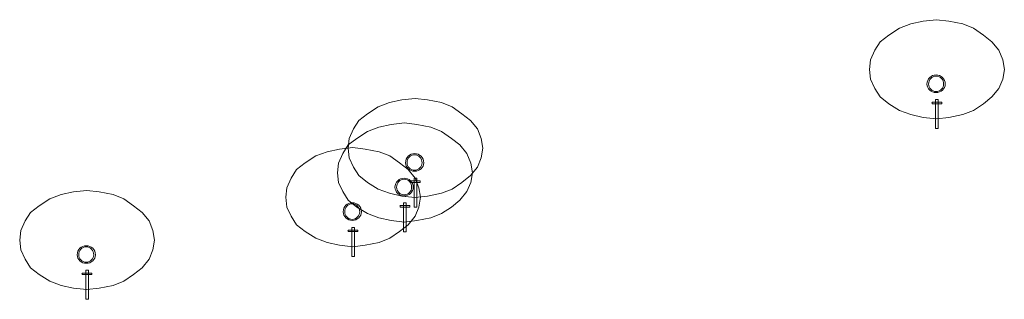
# Model space of a CAD drawing. Units: inches. Extents: x 22042254 to 25404563, y 17568978 to 17626777.
# Tile 45 of 45: x 25402992 to 25404563, y 17598821 to 17599268. Entities that reach past the tile are written whole.
import ezdxf

# ---------------------------------------------------------------- set-up
doc = ezdxf.new("R2010")
doc.units = ezdxf.units.IN
doc.header["$MEASUREMENT"] = 0
doc.layers.add('PLUMBING FIXTURES', color=9, linetype='Continuous', lineweight=18)

# ---------------------------------------------------------------- blocks, each defined once
blk = doc.blocks.new('WASH')
for p, q in [((268674.25, -2306.86), (268674.25, -2306.65)), ((268674.71, -2306.29), (268675.07, -2306.29)), ((268675.53, -2306.86), (268675.53, -2306.65)), ((268674.71, -2310.15), (268675.07, -2310.15))]:
    blk.add_line(p, q)
for points in [[(268665.93, -2302.29), (268666.07, -2301.01), (268666.64, -2299.72), (268667.36, -2298.58), (268668.5, -2297.72), (268669.93, -2296.79), (268671.43, -2296.22), (268673.07, -2295.86), (268674.86, -2295.65), (268676.5, -2295.86), (268678.36, -2296.22), (268679.78, -2296.79), (268681.07, -2297.72), (268682.21, -2298.58), (268683.14, -2299.72), (268683.64, -2301.01), (268683.86, -2302.29), (268683.64, -2303.58), (268683.14, -2304.79), (268682.21, -2305.94), (268681.07, -2306.86), (268679.78, -2307.72), (268678.36, -2308.29), (268676.5, -2308.65), (268674.86, -2308.86), (268673.07, -2308.65), (268671.43, -2308.29), (268669.93, -2307.72), (268668.5, -2306.86), (268667.36, -2305.94), (268666.64, -2304.79), (268666.07, -2303.58)], [(268674.14, -2306.65), (268674.14, -2306.65)], [(268674.86, -2306.29), (268674.86, -2306.29)], [(268675.43, -2306.65), (268675.43, -2306.65)]]:
    blk.add_lwpolyline(points, close=True)
for points in [[(268674.25, -2306.65), (268675.53, -2306.65), (268675.53, -2306.65)], [(268674.25, -2306.86), (268675.53, -2306.86), (268675.53, -2306.86)], [(268674.71, -2310.15), (268674.71, -2306.29), (268674.71, -2306.29)], [(268675.07, -2310.15), (268675.07, -2306.29), (268675.07, -2306.29)]]:
    blk.add_lwpolyline(points)
for points in [[(268673.57, -2304.22), (268673.57, -2304.86), (268674.14, -2305.36), (268674.78, -2305.36), (268674.78, -2305.36), (268675.43, -2305.36), (268676, -2304.86), (268676, -2304.22), (268676, -2304.22), (268676, -2303.51), (268675.43, -2303.01), (268674.78, -2303.01), (268674.78, -2303.01), (268674.14, -2303.01), (268673.57, -2303.51), (268673.57, -2304.22)], [(268673.78, -2304.22), (268673.78, -2304.72), (268674.21, -2305.22), (268674.78, -2305.22), (268674.78, -2305.22), (268675.36, -2305.22), (268675.78, -2304.72), (268675.78, -2304.22), (268675.78, -2304.22), (268675.78, -2303.65), (268675.36, -2303.15), (268674.78, -2303.15), (268674.78, -2303.15), (268674.21, -2303.15), (268673.78, -2303.65), (268673.78, -2304.22)]]:
    blk.add_open_spline(points, degree=3, knots=[0, 0, 0, 0, 0.0625, 0.0625, 0.0625, 0.062501, 0.125, 0.125, 0.125, 0.125001, 0.1875, 0.1875, 0.1875, 0.187501, 1, 1, 1, 1])

msp = doc.modelspace()

# ---------------------------------------------------------------- block references
at = {"layer": 'PLUMBING FIXTURES', "xscale": 12, "yscale": 12, "zscale": 12}
for p in [(22180357.151, 17626815.762), (22179524.979, 17626690.125), (22179508.168, 17626650.935), (22179425.511, 17626611.745), (22179001.02, 17626543.162)]:
    msp.add_blockref('WASH', p, dxfattribs=at)

doc.saveas('drawing.dxf')
